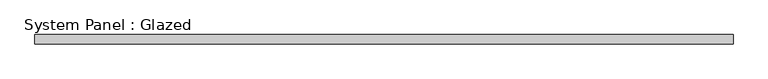
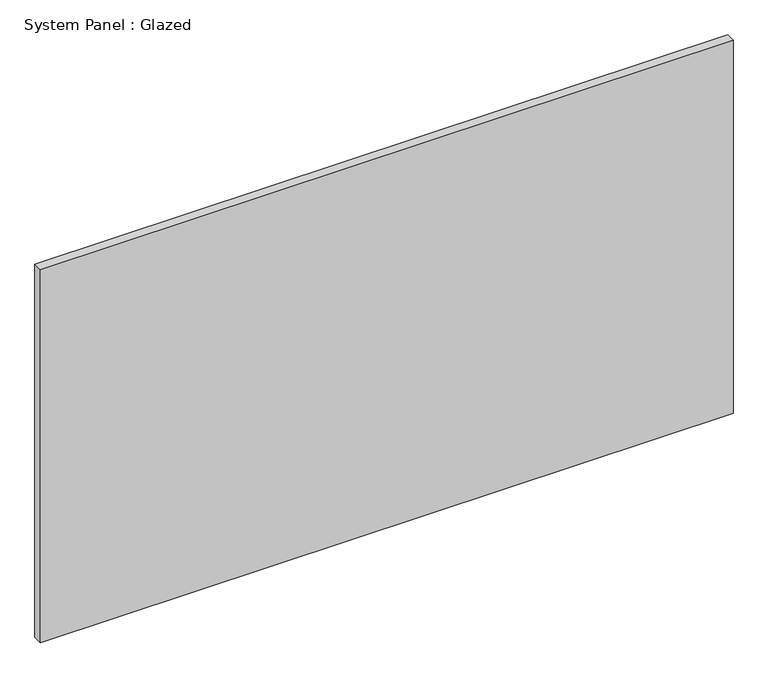
"""IFC4 building model written with IfcOpenShell, lengths in millimetres: plate geometry, System Panel : Glazed."""

from ifc_helpers import new_model, si_unit, origin, origin_with_axes, place, context, project, spatial, polyline, outline, extrude, source, transform, mapped, element, save


def system_panel_glazed_3dcdd35b(model_context):
    return source(origin(), model_context, "Body", "SweptSolid", [
        extrude(outline(polyline([(915.0000002, 24.5), (-915.0000002, 24.5), (-915.0000002, 49.5), (915.0000002, 49.5), (915.0000002, 24.5)])), origin_with_axes(), (0.0, 0.0, 1.0), 1041.4),
    ])


if __name__ == "__main__":
    model = new_model("IFC4")
    model_context = context("Model", 3, world=origin())
    ifc_project = project(units=[si_unit("LENGTHUNIT", "METRE", prefix="MILLI")], contexts=[model_context])
    site = spatial("IfcSite", under=ifc_project)
    building = spatial("IfcBuilding", under=site)
    placement = place(None, origin())
    system_panel_glazed_shape = system_panel_glazed_3dcdd35b(model_context)
    element("IfcPlate", 1, ObjectType="System Panel : Glazed", at=placement, inside=building, context=model_context, shape_type="MappedRepresentation", body=[
        mapped(system_panel_glazed_shape, transform((0.0, 0.0, 0.0), x_axis=(1.0, 0.0, 0.0), y_axis=(0.0, 1.0, 0.0), z_axis=(0.0, 0.0, 1.0))),
    ])
    save(model, "model.ifc")

# Revit data of these elements
# Type "System Panel : Glazed"
#   Keynote = "H11"
#   Construction Type Id = "GSP4R"
#   Analytic Construction = "1/8 in Pilkington single glazing"
#   Visual Light Transmittance = 0.9
#   Solar Heat Gain Coefficient = 0.86
#   Heat Transfer Coefficient (U) = 6.7069 W/(m²·K)
#   Define Thermal Properties by = 1
# Element 1 (IfcPlate, "System Panel : Glazed")
#   Materials on its faces: "Glass"
# Materials
#   "Glass": class "Glass", colour RGB 0 128 192, transparency 0.9, Description = "Soda Lime Glass", Cost = 0
